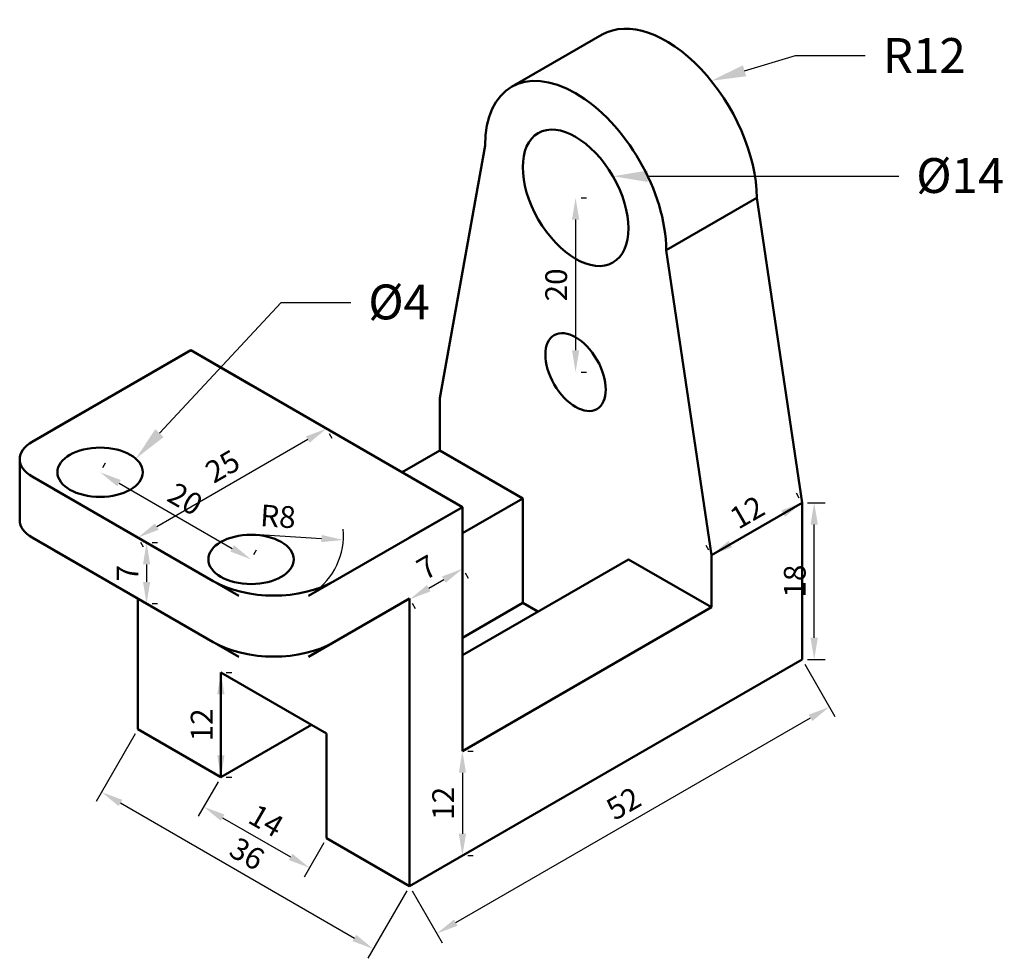
# Model space of a CAD drawing. Units: millimetres. Extents: x 2114 to 2227, y 1667 to 1774.
import ezdxf
from ezdxf import colors
from ezdxf.entities.mleader import LeaderData, LeaderLine
from ezdxf.math import Vec2, Vec3

# ---------------------------------------------------------------- set-up
doc = ezdxf.new("R2010")
doc.units = ezdxf.units.MM
doc.layers.add('M-DIMS', color=2, linetype='Continuous', lineweight=25)
doc.layers.add('M-OUTL', color=7, linetype='Continuous', lineweight=50)
doc.styles.get("Standard").update_dxf_attribs({"font": 'arial.ttf'})
doc.dimstyles.new('ISO-25', dxfattribs={"dimtxt": 2.5, "dimasz": 2.5, "dimexe": 1.25, "dimexo": 0.625, "dimtad": 1, "dimtxsty": 'Standard', "dimcen": 2.5, "dimadec": 0, "dimazin": 0, "dimtfac": 1, "dimtmove": 0, "dimatfit": 3, "dimfxl": 1, "dimarcsym": 0})

# ---------------------------------------------------------------- blocks, each defined once
blk = doc.blocks.new('*D1')
at = {"layer": 'Defpoints', "color": 0, "transparency": 16777216}
for p in [(2204.24, 1700.79), (2207.38, 1695.35), (2159.21, 1674.79)]:
    blk.add_point(p, dxfattribs=at)
at = {"layer": 'M-DIMS', "color": 0, "lineweight": -2, "transparency": 16777216}
for p, q in [((2204.56, 1700.25), (2208.01, 1694.27)), ((2164.51, 1670.6), (2205.22, 1694.1)), ((2159.52, 1674.25), (2162.97, 1668.27))]:
    blk.add_line(p, q, dxfattribs=at)
at = {"layer": 'M-DIMS', "color": 0, "transparency": 16777216}
for points in [[(2205.01, 1694.46), (2205.43, 1693.74), (2207.38, 1695.35)], [(2164.31, 1670.96), (2164.72, 1670.24), (2162.35, 1669.35)]]:
    blk.add_solid(points, dxfattribs=at)
at = {"layer": 'M-DIMS', "color": 0, "transparency": 16777216, "insert": (2183.92, 1684), "char_height": 2.5, "attachment_point": 5, "rotation": 30}
blk.add_mtext('52', dxfattribs=at)
blk = doc.blocks.new('*D2')
at = {"layer": 'Defpoints', "color": 0, "transparency": 16777216}
for p in [(2165.27, 1690.29), (2165.27, 1678.29), (2165.27, 1678.29)]:
    blk.add_point(p, dxfattribs=at)
at = {"layer": 'M-DIMS', "color": 0, "lineweight": -2, "transparency": 16777216}
for p, q in [((2165.9, 1690.29), (2166.52, 1690.29)), ((2165.27, 1687.79), (2165.27, 1680.79)), ((2165.9, 1678.29), (2166.52, 1678.29))]:
    blk.add_line(p, q, dxfattribs=at)
at = {"layer": 'M-DIMS', "color": 0, "transparency": 16777216}
for points in [[(2164.86, 1687.79), (2165.69, 1687.79), (2165.27, 1690.29)], [(2164.86, 1680.79), (2165.69, 1680.79), (2165.27, 1678.29)]]:
    blk.add_solid(points, dxfattribs=at)
at = {"layer": 'M-DIMS', "color": 0, "transparency": 16777216, "insert": (2163.39, 1684.29), "char_height": 2.5, "attachment_point": 5, "rotation": 90}
blk.add_mtext('12', dxfattribs=at)
blk = doc.blocks.new('*D3')
at = {"layer": 'Defpoints', "color": 0, "transparency": 16777216}
for p in [(2165.27, 1711.29), (2165.31, 1711.22), (2159.21, 1707.79)]:
    blk.add_point(p, dxfattribs=at)
at = {"layer": 'M-DIMS', "color": 0, "lineweight": -2, "transparency": 16777216}
for p, q in [((2165.58, 1710.75), (2165.94, 1710.14)), ((2161.41, 1708.97), (2163.14, 1709.97)), ((2159.52, 1707.25), (2159.87, 1706.64))]:
    blk.add_line(p, q, dxfattribs=at)
at = {"layer": 'M-DIMS', "color": 0, "transparency": 16777216}
for points in [[(2162.94, 1710.33), (2163.35, 1709.61), (2165.31, 1711.22)], [(2161.2, 1709.33), (2161.62, 1708.61), (2159.25, 1707.72)]]:
    blk.add_solid(points, dxfattribs=at)
at = {"layer": 'M-DIMS', "color": 0, "transparency": 16777216, "insert": (2161.34, 1711.1), "char_height": 2.5, "attachment_point": 5, "rotation": 30}
blk.add_mtext('7', dxfattribs=at)
blk = doc.blocks.new('*D4')
at = {"layer": 'Defpoints', "color": 0, "transparency": 16777216}
for p in [(2129.03, 1714.21), (2129.03, 1707.21), (2129.03, 1707.21)]:
    blk.add_point(p, dxfattribs=at)
at = {"layer": 'M-DIMS', "color": 0, "lineweight": -2, "transparency": 16777216}
for p, q in [((2129.66, 1714.21), (2130.28, 1714.21)), ((2129.03, 1711.71), (2129.03, 1709.71)), ((2129.66, 1707.21), (2130.28, 1707.21))]:
    blk.add_line(p, q, dxfattribs=at)
at = {"layer": 'M-DIMS', "color": 0, "transparency": 16777216}
for points in [[(2128.62, 1711.71), (2129.45, 1711.71), (2129.03, 1714.21)], [(2128.62, 1709.71), (2129.45, 1709.71), (2129.03, 1707.21)]]:
    blk.add_solid(points, dxfattribs=at)
at = {"layer": 'M-DIMS', "color": 0, "transparency": 16777216, "insert": (2127.16, 1710.71), "char_height": 2.5, "attachment_point": 5, "rotation": 90}
blk.add_mtext('7', dxfattribs=at)
blk = doc.blocks.new('*D5')
at = {"layer": 'Defpoints', "color": 0, "transparency": 16777216}
for p in [(2204.24, 1718.79), (2204.24, 1718.79), (2193.85, 1712.79)]:
    blk.add_point(p, dxfattribs=at)
at = {"layer": 'M-DIMS', "color": 0, "lineweight": -2, "transparency": 16777216}
for p, q in [((2203.93, 1719.33), (2203.62, 1719.87)), ((2196.02, 1714.04), (2202.08, 1717.54)), ((2193.54, 1713.33), (2193.23, 1713.87))]:
    blk.add_line(p, q, dxfattribs=at)
at = {"layer": 'M-DIMS', "color": 0, "transparency": 16777216}
for points in [[(2201.87, 1717.9), (2202.29, 1717.18), (2204.24, 1718.79)], [(2195.81, 1714.4), (2196.22, 1713.68), (2193.85, 1712.79)]]:
    blk.add_solid(points, dxfattribs=at)
at = {"layer": 'M-DIMS', "color": 0, "transparency": 16777216, "insert": (2198.11, 1717.42), "char_height": 2.5, "attachment_point": 5, "rotation": 30}
blk.add_mtext('12', dxfattribs=at)
blk = doc.blocks.new('*D6')
at = {"layer": 'Defpoints', "color": 0, "transparency": 16777216}
for p in [(2204.24, 1718.79), (2205.64, 1718.79), (2204.24, 1700.79)]:
    blk.add_point(p, dxfattribs=at)
at = {"layer": 'M-DIMS', "color": 0, "lineweight": -2, "transparency": 16777216}
for p, q in [((2204.87, 1718.79), (2206.89, 1718.79)), ((2205.64, 1703.29), (2205.64, 1716.29)), ((2204.87, 1700.79), (2206.89, 1700.79))]:
    blk.add_line(p, q, dxfattribs=at)
at = {"layer": 'M-DIMS', "color": 0, "transparency": 16777216}
for points in [[(2205.22, 1716.29), (2206.06, 1716.29), (2205.64, 1718.79)], [(2205.22, 1703.29), (2206.06, 1703.29), (2205.64, 1700.79)]]:
    blk.add_solid(points, dxfattribs=at)
at = {"layer": 'M-DIMS', "color": 0, "transparency": 16777216, "insert": (2203.74, 1709.79), "char_height": 2.5, "attachment_point": 5, "rotation": 90}
blk.add_mtext('18', dxfattribs=at)
blk = doc.blocks.new('*D7')
at = {"layer": 'Defpoints', "color": 0, "transparency": 16777216}
for p in [(2128.03, 1692.79), (2159.21, 1674.79), (2155.05, 1667.58)]:
    blk.add_point(p, dxfattribs=at)
at = {"layer": 'M-DIMS', "color": 0, "lineweight": -2, "transparency": 16777216}
for p, q in [((2127.72, 1692.25), (2123.25, 1684.5)), ((2126.04, 1684.33), (2152.88, 1668.83)), ((2158.9, 1674.25), (2154.42, 1666.5))]:
    blk.add_line(p, q, dxfattribs=at)
at = {"layer": 'M-DIMS', "color": 0, "transparency": 16777216}
for points in [[(2126.25, 1684.69), (2125.83, 1683.97), (2123.87, 1685.58)], [(2153.09, 1669.19), (2152.68, 1668.47), (2155.05, 1667.58)]]:
    blk.add_solid(points, dxfattribs=at)
at = {"layer": 'M-DIMS', "color": 0, "transparency": 16777216, "insert": (2140.41, 1678.23), "char_height": 2.5, "attachment_point": 5, "rotation": 330}
blk.add_mtext('36', dxfattribs=at)
blk = doc.blocks.new('*D8')
at = {"layer": 'Defpoints', "color": 0, "transparency": 16777216}
for p in [(2137.56, 1687.29), (2149.68, 1680.29), (2147.72, 1676.89)]:
    blk.add_point(p, dxfattribs=at)
at = {"layer": 'M-DIMS', "color": 0, "lineweight": -2, "transparency": 16777216}
for p, q in [((2137.25, 1686.75), (2134.97, 1682.81)), ((2137.76, 1682.64), (2145.56, 1678.14)), ((2149.37, 1679.75), (2147.1, 1675.81))]:
    blk.add_line(p, q, dxfattribs=at)
at = {"layer": 'M-DIMS', "color": 0, "transparency": 16777216}
for points in [[(2137.97, 1683), (2137.56, 1682.28), (2135.6, 1683.89)], [(2145.77, 1678.5), (2145.35, 1677.78), (2147.72, 1676.89)]]:
    blk.add_solid(points, dxfattribs=at)
at = {"layer": 'M-DIMS', "color": 0, "transparency": 16777216, "insert": (2142.6, 1682.02), "char_height": 2.5, "attachment_point": 5, "rotation": 330}
blk.add_mtext('14', dxfattribs=at)
blk = doc.blocks.new('*D9')
at = {"layer": 'Defpoints', "color": 0, "transparency": 16777216}
for p in [(2137.56, 1699.29), (2137.56, 1687.29), (2137.56, 1687.29)]:
    blk.add_point(p, dxfattribs=at)
at = {"layer": 'M-DIMS', "color": 0, "lineweight": -2, "transparency": 16777216}
for p, q in [((2138.18, 1699.29), (2138.81, 1699.29)), ((2137.56, 1696.79), (2137.56, 1689.79)), ((2138.18, 1687.29), (2138.81, 1687.29))]:
    blk.add_line(p, q, dxfattribs=at)
at = {"layer": 'M-DIMS', "color": 0, "transparency": 16777216}
for points in [[(2137.14, 1696.79), (2137.98, 1696.79), (2137.56, 1699.29)], [(2137.14, 1689.79), (2137.98, 1689.79), (2137.56, 1687.29)]]:
    blk.add_solid(points, dxfattribs=at)
at = {"layer": 'M-DIMS', "color": 0, "transparency": 16777216, "insert": (2135.68, 1693.29), "char_height": 2.5, "attachment_point": 5, "rotation": 90}
blk.add_mtext('12', dxfattribs=at)
blk = doc.blocks.new('*D10')
at = {"layer": 'Defpoints', "color": 0, "transparency": 16777216}
for p in [(2178.26, 1753.79), (2178.26, 1733.79), (2178.26, 1733.79)]:
    blk.add_point(p, dxfattribs=at)
at = {"layer": 'M-DIMS', "color": 0, "lineweight": -2, "transparency": 16777216}
for p, q in [((2178.89, 1753.79), (2179.51, 1753.79)), ((2178.26, 1751.29), (2178.26, 1736.29)), ((2178.89, 1733.79), (2179.51, 1733.79))]:
    blk.add_line(p, q, dxfattribs=at)
at = {"layer": 'M-DIMS', "color": 0, "transparency": 16777216}
for points in [[(2177.85, 1751.29), (2178.68, 1751.29), (2178.26, 1753.79)], [(2177.85, 1736.29), (2178.68, 1736.29), (2178.26, 1733.79)]]:
    blk.add_solid(points, dxfattribs=at)
at = {"layer": 'M-DIMS', "color": 0, "transparency": 16777216, "insert": (2176.36, 1743.79), "char_height": 2.5, "attachment_point": 5, "rotation": 90}
blk.add_mtext('20', dxfattribs=at)
blk = doc.blocks.new('*D11')
at = {"layer": 'Defpoints', "color": 0, "transparency": 16777216}
for p in [(2123.7, 1722.29), (2141.02, 1712.29), (2141.02, 1712.29)]:
    blk.add_point(p, dxfattribs=at)
at = {"layer": 'M-DIMS', "color": 0, "lineweight": -2, "transparency": 16777216}
for p, q in [((2124.02, 1722.83), (2124.33, 1723.37)), ((2125.87, 1721.04), (2138.86, 1713.54)), ((2141.34, 1712.83), (2141.65, 1713.37))]:
    blk.add_line(p, q, dxfattribs=at)
at = {"layer": 'M-DIMS', "color": 0, "transparency": 16777216}
for points in [[(2126.08, 1721.4), (2125.66, 1720.68), (2123.7, 1722.29)], [(2139.07, 1713.9), (2138.65, 1713.18), (2141.02, 1712.29)]]:
    blk.add_solid(points, dxfattribs=at)
at = {"layer": 'M-DIMS', "color": 0, "transparency": 16777216, "insert": (2133.31, 1718.94), "char_height": 2.5, "attachment_point": 5, "rotation": 330}
blk.add_mtext('20', dxfattribs=at)
blk = doc.blocks.new('*D12')
at = {"layer": 'Defpoints', "color": 0, "transparency": 16777216}
for p in [(2143.62, 1715.03), (2151.61, 1714.52)]:
    blk.add_point(p, dxfattribs=at)
at = {"layer": 'M-DIMS', "color": 0, "lineweight": -2, "transparency": 16777216}
blk.add_line((2141.34, 1715.17), (2149.11, 1714.68), dxfattribs=at)
blk.add_arc((2143.62, 1715.03), 8, 304.4762, 5.3029, dxfattribs=at)
at = {"layer": 'M-DIMS', "color": 0, "transparency": 16777216}
blk.add_solid([(2149.14, 1715.09), (2149.08, 1714.26), (2151.61, 1714.52)], dxfattribs=at)
at = {"layer": 'M-DIMS', "color": 0, "transparency": 16777216, "insert": (2144.1, 1716.9), "char_height": 2.5, "attachment_point": 5, "rotation": 356.3505}
blk.add_mtext('R8', dxfattribs=at)
blk = doc.blocks.new('*D13')
at = {"layer": 'Defpoints', "color": 0, "transparency": 16777216}
for p in [(2149.68, 1727.29), (2128.03, 1714.79), (2128.03, 1714.79)]:
    blk.add_point(p, dxfattribs=at)
at = {"layer": 'M-DIMS', "color": 0, "lineweight": -2, "transparency": 16777216}
for p, q in [((2150, 1726.75), (2150.31, 1726.21)), ((2147.52, 1726.04), (2130.2, 1716.04)), ((2128.35, 1714.25), (2128.66, 1713.71))]:
    blk.add_line(p, q, dxfattribs=at)
at = {"layer": 'M-DIMS', "color": 0, "transparency": 16777216}
for points in [[(2147.31, 1726.4), (2147.73, 1725.68), (2149.68, 1727.29)], [(2129.99, 1716.4), (2130.41, 1715.68), (2128.03, 1714.79)]]:
    blk.add_solid(points, dxfattribs=at)
at = {"layer": 'M-DIMS', "color": 0, "transparency": 16777216, "insert": (2137.91, 1722.69), "char_height": 2.5, "attachment_point": 5, "rotation": 30}
blk.add_mtext('25', dxfattribs=at)

msp = doc.modelspace()

# ---------------------------------------------------------------- linework, layer by layer
at = {"layer": 'M-OUTL'}
for p, q in [((2170.914, 1766.516), (2181.306, 1772.516)), ((2167.87, 1759.788), (2162.674, 1730.788)), ((2188.655, 1747.788), (2199.047, 1753.788)), ((2199.047, 1753.788), (2204.243, 1718.788)), ((2188.655, 1747.788), (2193.851, 1712.788)), ((2115.909, 1725.788), (2134.095, 1736.288)), ((2134.095, 1736.288), (2118.445, 1727.253)), ((2128.033, 1732.788), (2134.095, 1736.288)), ((2134.095, 1736.288), (2165.272, 1718.288)), ((2134.095, 1736.288), (2141.023, 1732.288)), ((2162.674, 1730.788), (2162.674, 1724.788)), ((2162.674, 1724.788), (2158.344, 1722.288)), ((2162.674, 1724.788), (2172.2, 1719.288)), ((2114.474, 1723.788), (2114.474, 1716.788)), ((2115.909, 1721.788), (2136.693, 1709.788)), ((2118.445, 1720.324), (2139.621, 1708.098)), ((2118.507, 1720.288), (2118.445, 1720.253)), ((2172.2, 1719.288), (2165.272, 1715.288)), ((2172.2, 1719.288), (2172.2, 1707.288)), ((2204.243, 1718.788), (2193.851, 1712.788)), ((2204.243, 1700.788), (2204.243, 1718.788)), ((2147.621, 1708.098), (2165.272, 1718.288)), ((2159.21, 1714.788), (2165.272, 1718.288)), ((2165.272, 1690.288), (2165.272, 1718.288)), ((2115.909, 1714.788), (2136.693, 1702.788)), ((2118.445, 1713.324), (2139.621, 1701.098)), ((2184.325, 1712.288), (2165.272, 1701.288)), ((2193.851, 1706.788), (2184.325, 1712.288)), ((2193.851, 1712.788), (2193.851, 1706.788)), ((2128.033, 1692.788), (2128.033, 1707.788)), ((2147.621, 1701.098), (2159.21, 1707.788)), ((2159.21, 1674.788), (2159.21, 1707.788)), ((2165.272, 1703.288), (2172.2, 1707.288)), ((2172.2, 1707.288), (2173.932, 1706.288)), ((2193.851, 1706.788), (2165.272, 1690.288)), ((2159.21, 1674.788), (2204.243, 1700.788)), ((2137.559, 1687.288), (2137.559, 1699.288)), ((2137.559, 1699.288), (2149.684, 1692.288)), ((2128.033, 1692.788), (2137.559, 1687.288)), ((2137.559, 1687.288), (2147.952, 1693.288)), ((2149.684, 1692.288), (2149.684, 1680.288)), ((2149.684, 1680.288), (2159.21, 1674.788))]:
    msp.add_line(p, q, dxfattribs=at)
for centre, major_axis, start_param, end_param in [((2188.655, 1759.788), (7.348, -12.728), 7.0685835, 9.424778), ((2178.262, 1753.788), (7.348, -12.728), 0.7853982, 3.9269908), ((2119.373, 1723.788), (4.899, 0), 2.3561946, 3.1415927), ((2119.373, 1723.788), (4.899, 0), 3.1415927, 3.9269907), ((2119.373, 1716.788), (4.899, 0), 3.1415927, 3.9269907), ((2143.621, 1713.788), (9.798, 0), 3.9269909, 5.497787), ((2143.621, 1706.788), (9.798, 0), 3.9269909, 5.497787)]:
    msp.add_ellipse(centre, major_axis=major_axis, ratio=0.5773503, start_param=start_param, end_param=end_param, dxfattribs=at)
for centre, major_axis in [((2178.262, 1753.788), (4.287, -7.425)), ((2178.262, 1733.788), (2.449, -4.243)), ((2123.703, 1722.288), (-4.899, 0)), ((2141.023, 1712.288), (-4.899, 0))]:
    msp.add_ellipse(centre, major_axis=major_axis, ratio=0.5773503, dxfattribs=at)

# ---------------------------------------------------------------- dimensions: what is measured, and where the dimension line sits
at = {"layer": 'M-DIMS'}
for p1, p2, distance, picture, middle in [((2178.262, 1753.788), (2178.262, 1733.788), 0, '*D10', (2176.361, 1743.788)), ((2149.684, 1727.288), (2128.033, 1714.788), 0, '*D13', (2137.908, 1722.685)), ((2123.703, 1722.288), (2141.023, 1712.288), 0, '*D11', (2133.314, 1718.935)), ((2193.851, 1712.788), (2204.243, 1718.788), 0, '*D5', (2198.107, 1717.417)), ((2204.243, 1700.788), (2204.243, 1718.788), -1.395, '*D6', (2203.737, 1709.788)), ((2129.033, 1714.211), (2129.033, 1707.211), 0, '*D4', (2127.158, 1710.711)), ((2159.21, 1707.788), (2165.272, 1711.288), -0.076, '*D3', (2161.341, 1711.096)), ((2159.21, 1674.788), (2204.243, 1700.788), -6.279, '*D1', (2183.915, 1683.998)), ((2137.559, 1699.288), (2137.559, 1687.288), 0, '*D9', (2135.679, 1693.288)), ((2128.033, 1692.788), (2159.21, 1674.788), -8.32, '*D7', (2140.413, 1678.23)), ((2165.272, 1690.288), (2165.272, 1678.288), 0, '*D2', (2163.392, 1684.288)), ((2137.559, 1687.288), (2149.684, 1680.288), -3.92, '*D8', (2142.602, 1682.022))]:
    dim = msp.add_aligned_dim(p1=p1, p2=p2, distance=distance, dimstyle='ISO-25', override={"dimclrd": 0, "dimclre": 0, "dimclrt": 0}, dxfattribs=at)
    dim.commit()
    dim.dimension.update_dxf_attribs({"geometry": picture, "text_midpoint": middle})
dim = msp.add_radius_dim(center=(2143.621, 1715.026), mpoint=(2151.605, 1714.517), dimstyle='ISO-25', override={"dimclrd": 0, "dimclre": 0, "dimclrt": 0}, dxfattribs=at)
dim.commit()
dim.dimension.update_dxf_attribs({"geometry": '*D12', "text_midpoint": (2143.977, 1715.003), "dimtype": 164})

# ---------------------------------------------------------------- leaders
ml = msp.add_multileader_mtext('Standard', dxfattribs=at)
ml.set_content('R12', color=256)
ml.set_leader_properties()
ml.build(insert=Vec2(0, 0))
ctx = ml.context
ctx.base_point, ctx.plane_origin = Vec3(2211.507, 1770.121), Vec3(2193.821, 1767.218)
notes = []
notes.append((ctx, [(0, (1, 1, 0), (2203.507, 1770.121), (1, 0), 8, [(0, [(2193.821, 1767.218)], 0, [])])]))
ctx.mtext.insert, ctx.mtext.flow_direction = Vec3(2213.507, 1772.121), 5
ml = msp.add_multileader_mtext('Standard', dxfattribs=at)
ml.set_content('%%C14', color=256)
ml.set_leader_properties()
ml.build(insert=Vec2(0, 0))
ctx = ml.context
ctx.base_point, ctx.plane_origin = Vec3(2215.349, 1756.263), Vec3(2182.549, 1756.263)
notes.append((ctx, [(0, (1, 1, 0), (2207.349, 1756.263), (1, 0), 8, [(0, [(2182.549, 1756.263)], 0, [])])]))
ctx.mtext.insert, ctx.mtext.flow_direction = Vec3(2217.349, 1758.344), 5
ml = msp.add_multileader_mtext('Standard', dxfattribs=at)
ml.set_content('%%C4', color=256)
ml.set_leader_properties()
ml.build(insert=Vec2(0, 0))
ctx = ml.context
ctx.base_point, ctx.plane_origin = Vec3(2152.469, 1741.754), Vec3(2127.79, 1723.848)
notes.append((ctx, [(0, (1, 1, 0), (2144.469, 1741.754), (1, 0), 8, [(0, [(2127.79, 1723.848)], 0, [])])]))
ctx.mtext.insert, ctx.mtext.flow_direction = Vec3(2154.469, 1743.835), 5
for ctx, leaders in notes:
    for number, flags, end, landing, length, lines in leaders:
        leader = LeaderData()
        leader.index, (leader.has_last_leader_line, leader.has_dogleg_vector, leader.attachment_direction) = number, flags
        leader.last_leader_point, leader.dogleg_vector, leader.dogleg_length = Vec3(end), Vec3(landing), length
        for number, points, colour, breaks in lines:
            line = LeaderLine()
            line.index, line.vertices, line.color, line.breaks = number, Vec3.list(points), colors.encode_raw_color(colour), breaks
            leader.lines.append(line)
        ctx.leaders.append(leader)

doc.saveas('drawing.dxf')
